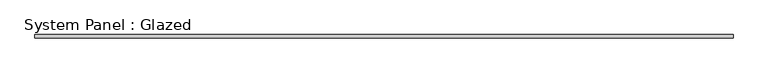
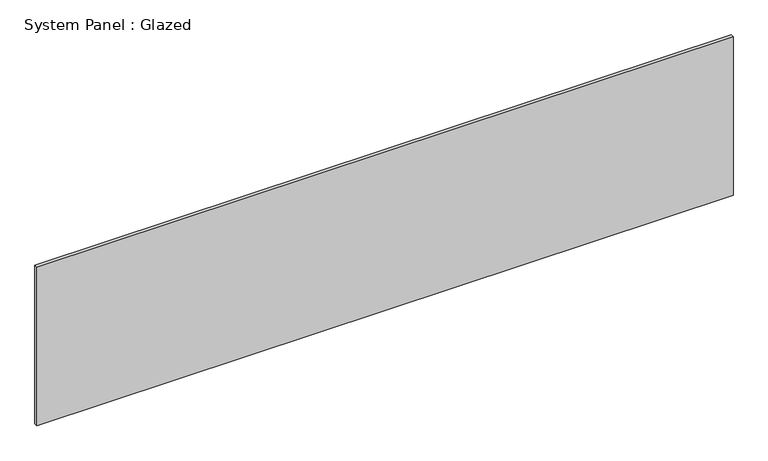
"""IFC4 building model written with IfcOpenShell, lengths in millimetres: plate geometry, System Panel : Glazed."""

from ifc_helpers import new_model, si_unit, origin, origin_with_axes, place, context, project, spatial, polyline, outline, extrude, source, transform, mapped, element, save


def system_panel_glazed_2dfb9705(model_context):
    return source(origin(), model_context, "Body", "SweptSolid", [
        extrude(outline(polyline([(2536.5851712, 19.05), (-2536.5851712, 19.05), (-2536.5851712, 44.45), (2536.5851712, 44.45), (2536.5851712, 19.05)])), origin_with_axes(), (0.0, 0.0, 1.0), 1219.2),
    ])


if __name__ == "__main__":
    model = new_model("IFC4")
    model_context = context("Model", 3, world=origin())
    ifc_project = project(units=[si_unit("LENGTHUNIT", "METRE", prefix="MILLI")], contexts=[model_context])
    site = spatial("IfcSite", under=ifc_project)
    building = spatial("IfcBuilding", under=site)
    placement = place(None, origin())
    system_panel_glazed_shape = system_panel_glazed_2dfb9705(model_context)
    element("IfcPlate", 1, ObjectType="System Panel : Glazed", at=placement, inside=building, context=model_context, shape_type="MappedRepresentation", body=[
        mapped(system_panel_glazed_shape, transform((0.0, 0.0, 0.0), x_axis=(1.0, 0.0, 0.0), y_axis=(0.0, 1.0, 0.0), z_axis=(0.0, 0.0, 1.0))),
    ])
    save(model, "model.ifc")

# Revit data of these elements
# Type "System Panel : Glazed"
#   Construction Type Id = "GSP4R"
#   Analytic Construction = "1/8 in Pilkington single glazing"
#   Visual Light Transmittance = 0.9
#   Solar Heat Gain Coefficient = 0.86
#   Heat Transfer Coefficient (U) = 1.18115 BTU/(h·ft²·°F)
# Element 1 (IfcPlate, "System Panel : Glazed")
#   Materials on its faces: "Glass"
# Materials
#   "Glass": class "Glass", colour RGB 0 128 192, transparency 0.75, Description = "Soda Lime Glass", Cost = 0
